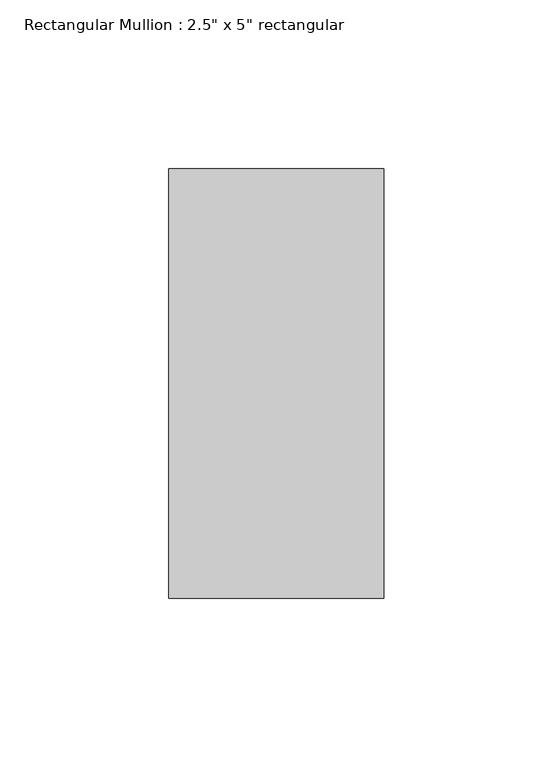
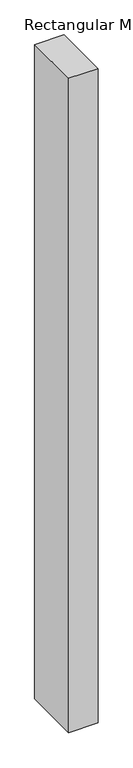
"""IFC4 building model written with IfcOpenShell, lengths in millimetres: member geometry."""

from ifc_helpers import new_model, si_unit, frame, origin, place, context, project, spatial, polyline, outline, extrude, source, transform, mapped, element, save


def member_6049e8cb(model_context):
    return source(origin(), model_context, "Body", "SweptSolid", [
        extrude(outline(polyline([(31.75, 63.5), (31.75, -63.5), (-31.75, -63.5), (-31.75, 63.5), (31.75, 63.5)])), frame((0.0, 0.0, -1493.5474484), z_axis=(0.0, 0.0, 1.0), x_axis=(1.0, 0.0, 0.0)), (0.0, 0.0, 1.0), 1493.5474484),
    ])


if __name__ == "__main__":
    model = new_model("IFC4")
    model_context = context("Model", 3, world=origin())
    ifc_project = project(units=[si_unit("LENGTHUNIT", "METRE", prefix="MILLI")], contexts=[model_context])
    site = spatial("IfcSite", under=ifc_project)
    building = spatial("IfcBuilding", under=site)
    placement = place(None, origin())
    member_shape = member_6049e8cb(model_context)
    element("IfcMember", 1, ObjectType="Rectangular Mullion : 2.5\" x 5\" rectangular", at=placement, inside=building, context=model_context, shape_type="MappedRepresentation", body=[
        mapped(member_shape, transform((0.0, 0.0, 0.0), x_axis=(1.0, 0.0, 0.0), y_axis=(0.0, 1.0, 0.0), z_axis=(0.0, 0.0, 1.0))),
    ])
    save(model, "model.ifc")

# Revit data of these elements
# Type "Rectangular Mullion : 2.5\" x 5\" rectangular"
#   built-in parameter 1007304 = 0.416667 (stored number, unit not read)
#   built-in parameter 1007301 = 0.104167 (stored number, unit not read)
#   built-in parameter 1007300 = 0.104167 (stored number, unit not read)
# Element 1 (IfcMember, "Rectangular Mullion : 2.5\" x 5\" rectangular")
#   Materials on its faces: "Aluminum"
# Materials
#   "Aluminum": class "Metal", colour RGB 247 247 247, transparency 0, Description = "Aluminum 6061", Cost = 0
